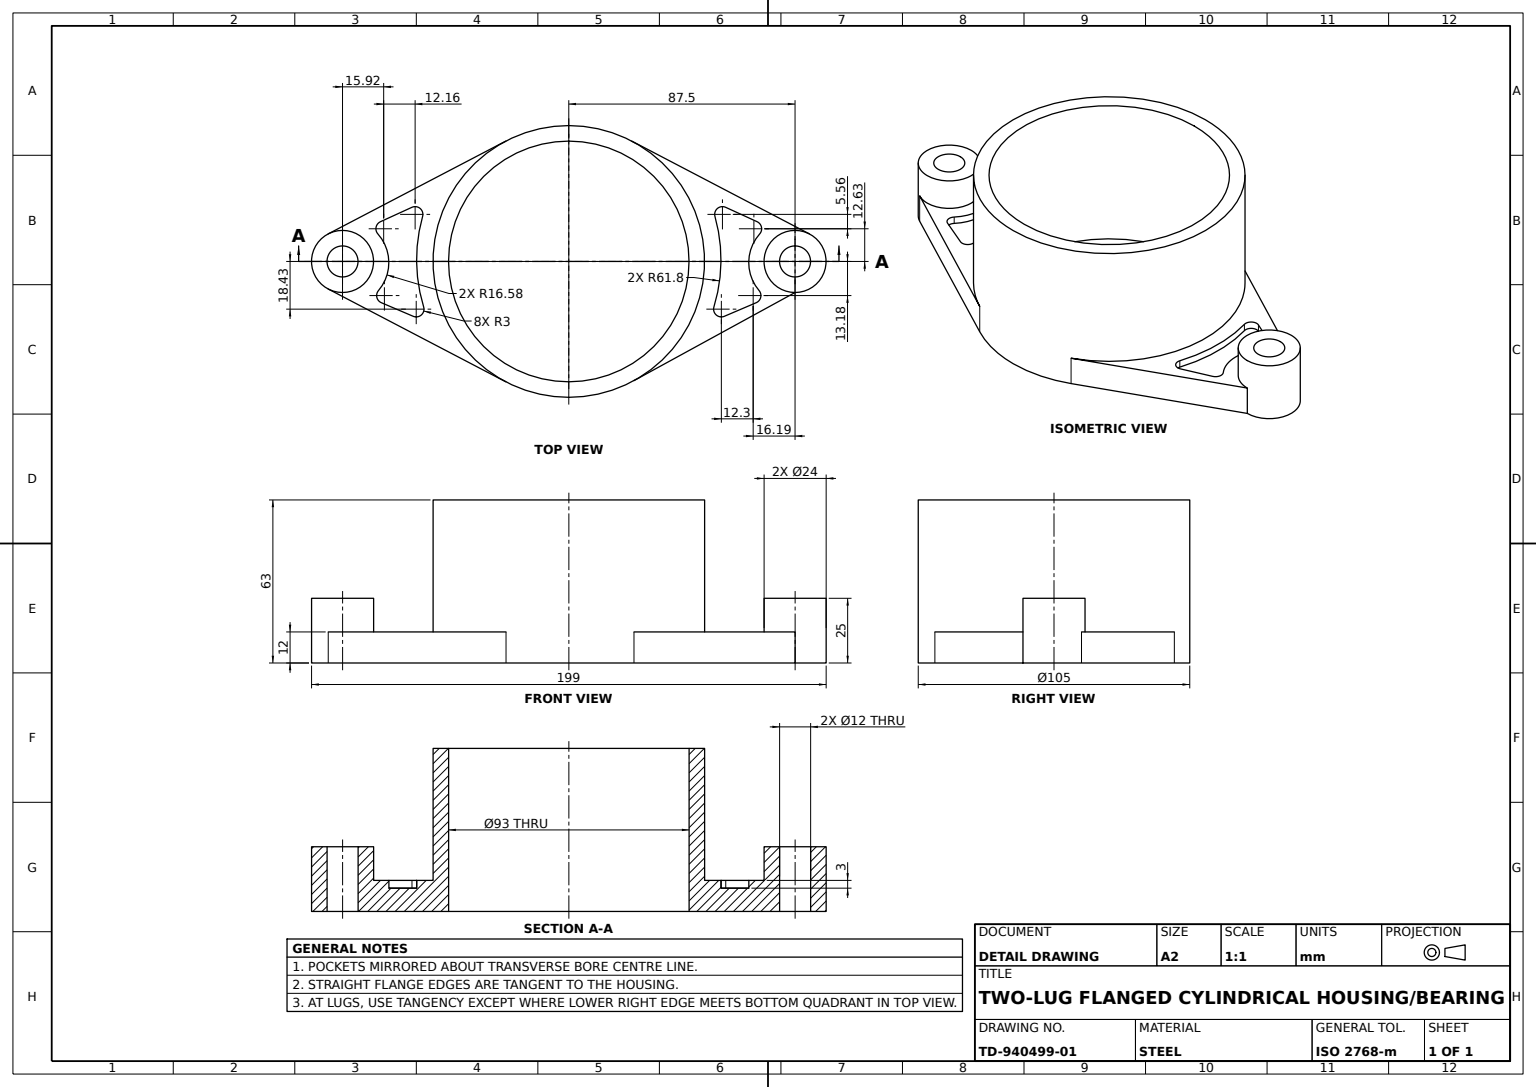
from build123d import *

# Parameters (mm, degrees)
HOUSING_BASE_PROFILE_SKETCH_R  = 52.5
HOUSING_CYLINDER_DEPTH         = 63
MOUNTING_FLANGE_DEPTH          = 12
SKETCH1_4_R                    = 12
LUG_BOSSES_DEPTH               = 25
BORE_AND_LUG_HOLES_SKETCH_R    = 6
BORE_AND_LUG_HOLES_SKETCH_R_2  = 46.5
BORE_AND_LUG_HOLES_2X_12_DEPTH = 129.939908485
FLANGE_RELIEF_POCKETS_DEPTH    = 3


with BuildPart() as part:
    # Housing Base Profile Sketch → Housing Cylinder (new body)
    with BuildSketch(Plane(origin=(0, 0, 0), x_dir=(1, 0, 0), z_dir=(0, 1, 0))):
        with Locations(Location((0, 0, 0), (0, 0, 270))):
            Circle(HOUSING_BASE_PROFILE_SKETCH_R)
    extrude(amount=HOUSING_CYLINDER_DEPTH)

    # Sketch1_3 → Mounting Flange (add)
    with BuildSketch(Plane(origin=(0, 0, 0), x_dir=(1, 0, 0), z_dir=(0, 1, 0))):
        with BuildLine():
            Line((-24.3, 46.537726631), (-93.054285714, 10.637194659))
            ThreePointArc((-93.054285714, 10.637194659), (-81.281134692, 10.262831689), (-75.5, 0))
            ThreePointArc((-75.5, 0), (-81.281134692, -10.262831689), (-93.054285714, -10.637194659))
            Line((-93.054285714, -10.637194659), (-24.3, -46.537726631))
            ThreePointArc((-24.3, -46.537726631), (-52.5, 0), (-24.3, 46.537726631))
        make_face()
        with BuildLine():
            Line((93.054285714, 10.637194659), (24.3, 46.537726631))
            ThreePointArc((24.3, 46.537726631), (44.899888641, 27.207535721), (52.5, 0))
            ThreePointArc((52.5, 0), (45.157075755, -26.778508346), (25.182342504, -46.066252572))
            Line((25.182342504, -46.066252572), (87.5, -12))
            ThreePointArc((87.5, -12), (75.845680288, 2.859516051), (93.054285714, 10.637194659))
        make_face()
    extrude(amount=MOUNTING_FLANGE_DEPTH)

    # Sketch1_4 → Lug Bosses (add)
    with BuildSketch(Plane(origin=(0, 0, 0), x_dir=(1, 0, 0), z_dir=(0, 1, 0))):
        with Locations(Location((87.5, 0, 0), (0, 0, 270))):
            Circle(SKETCH1_4_R)
        with Locations(Location((-87.5, 0, 0), (0, 0, 117.57162794))):
            Circle(SKETCH1_4_R)
    extrude(amount=LUG_BOSSES_DEPTH)

    # Bore and Lug Holes Sketch → Bore and Lug Holes 2x_12 (cut, through all)
    with BuildSketch(Plane(origin=(0, 63, 0), x_dir=(1, 0, 0), z_dir=(0, 1, 0))):
        with Locations(Location((-87.5, 0, 0), (0, 0, 270))):
            Circle(BORE_AND_LUG_HOLES_SKETCH_R)
        with Locations(Location((0, 0, 0), (0, 0, 270))):
            Circle(BORE_AND_LUG_HOLES_SKETCH_R_2)
        with Locations(Location((87.5, 0, 0), (0, 0, 270))):
            Circle(BORE_AND_LUG_HOLES_SKETCH_R)
    extrude(amount=-BORE_AND_LUG_HOLES_2X_12_DEPTH, mode=Mode.SUBTRACT)

    # Flange Pockets Sketch → Flange Relief Pockets (cut)
    with BuildSketch(Plane(origin=(0, 12, 0), x_dir=(1, 0, 0), z_dir=(0, 1, 0))):
        with BuildLine():
            Line((-60.67046514, 20.916189471), (-72.83224793, 15.355373632))
            ThreePointArc((-72.83224793, 15.355373632), (-74.521451253, 13.240091694), (-73.819589316, 10.625667214))
            ThreePointArc((-73.819589316, 10.625667214), (-69.591109503, -0.257419194), (-73.582978557, -11.22950162))
            ThreePointArc((-73.582978557, -11.22950162), (-74.226651592, -13.864622877), (-72.481931561, -15.941671512))
            Line((-72.481931561, -15.941671512), (-60.177135194, -21.187902521))
            ThreePointArc((-60.177135194, -21.187902521), (-56.993480479, -20.657990086), (-56.132769828, -17.547420732))
            ThreePointArc((-56.132769828, -17.547420732), (-58.852375063, -0.116051975), (-56.53564235, 17.373419684))
            ThreePointArc((-56.53564235, 17.373419684), (-57.471032791, 20.466004181), (-60.67046514, 20.916189471))
        make_face()
        with BuildLine():
            Line((60.67046514, 20.916189471), (72.83224793, 15.355373632))
            ThreePointArc((72.83224793, 15.355373632), (74.521451253, 13.240091694), (73.819589316, 10.625667214))
            ThreePointArc((73.819589316, 10.625667214), (69.591109503, -0.257419194), (73.582978557, -11.22950162))
            ThreePointArc((73.582978557, -11.22950162), (74.226651592, -13.864622877), (72.481931561, -15.941671512))
            Line((72.481931561, -15.941671512), (60.177135194, -21.187902521))
            ThreePointArc((60.177135194, -21.187902521), (56.993480479, -20.657990086), (56.132769828, -17.547420732))
            ThreePointArc((56.132769828, -17.547420732), (58.852375063, -0.116051975), (56.53564235, 17.373419684))
            ThreePointArc((56.53564235, 17.373419684), (57.471032791, 20.466004181), (60.67046514, 20.916189471))
        make_face()
    extrude(amount=-FLANGE_RELIEF_POCKETS_DEPTH, mode=Mode.SUBTRACT)


solid = part.part
